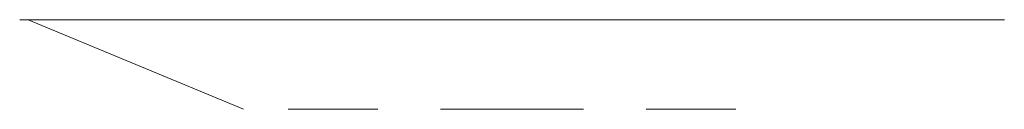
# Model space of a CAD drawing. Units: millimetres. Extents: x 61 to 171, y -10 to 0.
import ezdxf

# ---------------------------------------------------------------- set-up
doc = ezdxf.new("R2010")
doc.units = ezdxf.units.MM
doc.layers.add('M-CONS', color=8, linetype='Continuous', lineweight=18)

msp = doc.modelspace()

# ---------------------------------------------------------------- linework, layer by layer
at = {"layer": 'M-CONS', "extrusion": (0, -1, 0)}
for p, q in [((61.61, 0, 282.17), (87.31, 0, 356.73)), ((169.74, 0, 282.17), (144.04, 0, 356.73)), ((85.68, -10, 346.95), (61.61, 0, 282.17))]:
    msp.add_line(p, q, dxfattribs=at)
for centre, radius in [((75.68, 276.95), 15), ((75.68, 276.95), 15), ((75.68, 276.95), 10), ((115.68, 346.95), 30), ((155.68, 276.95), 15), ((155.68, 276.95), 10), ((95.68, 346.95, 10), 5), ((115.68, 346.95, 10), 8), ((115.68, 366.95, 10), 5), ((115.68, 326.95, 10), 5), ((135.68, 346.95, 10), 5)]:
    msp.add_circle(centre, radius, dxfattribs=at)
msp.add_arc((115.77, 215.57), 60, 63.1227, 117.1852, dxfattribs=at)

doc.saveas('drawing.dxf')
